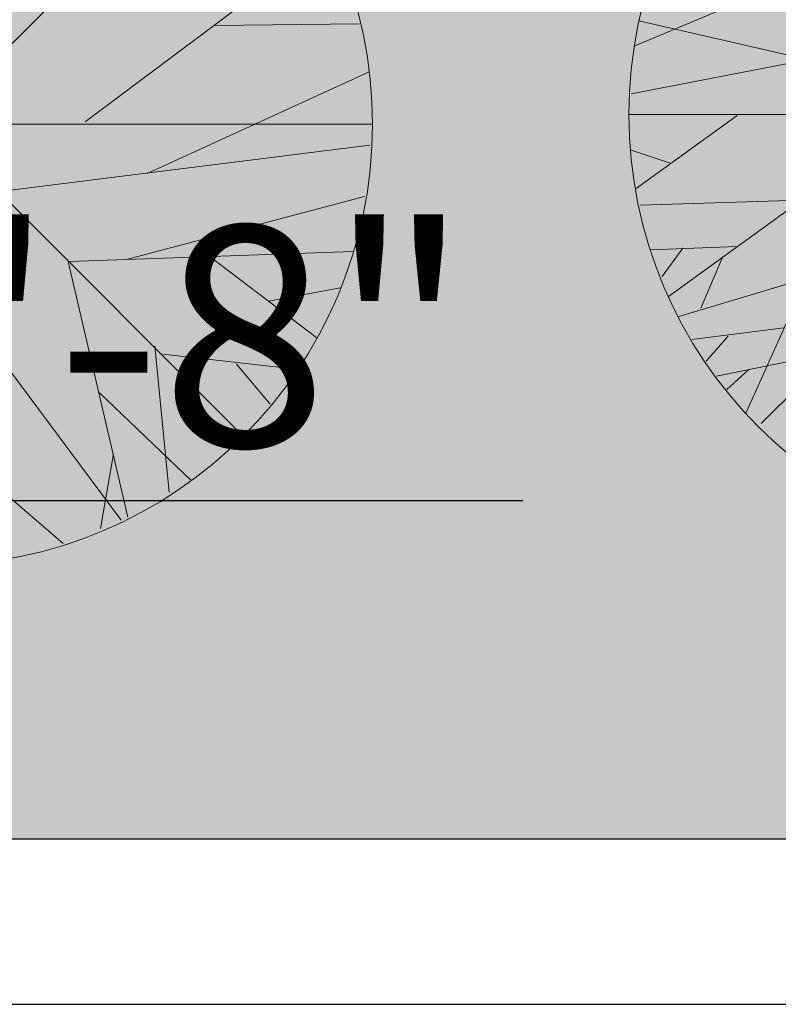
# Model space of a CAD drawing. Units: inches. Extents: x 459864 to 460310, y 324185 to 324787.
# Tile 57 of 112: x 460189 to 460210, y 324195 to 324222. Entities that reach past the tile are written whole.
import ezdxf

# ---------------------------------------------------------------- set-up
doc = ezdxf.new("R2010")
doc.units = ezdxf.units.IN
for name, color, linetype, lineweight in [('A-ANNO-DIMS', 2, 'Continuous', 18), ('C-PROP', 7, 'Continuous', 30), ('L-PLNT', 3, 'Continuous', 13), ('L-SITE-PATT', 252, 'Continuous', 13)]:
    doc.layers.add(name, color=color, linetype=linetype, lineweight=lineweight)
doc.styles.get("Standard").update_dxf_attribs({"font": 'arial.ttf'})
doc.dimstyles.new('ISO-25', dxfattribs={"dimtxt": 6, "dimasz": 2.5, "dimexe": 1.25, "dimexo": 0.625, "dimtad": 1, "dimdec": 1, "dimlunit": 3, "dimtxsty": 'Standard', "dimcen": 2.5, "dimadec": 0, "dimazin": 0, "dimtfac": 1, "dimtdec": 1, "dimtmove": 0, "dimatfit": 3, "dimfxl": 1, "dimarcsym": 0})

# ---------------------------------------------------------------- blocks, each defined once
blk = doc.blocks.new('Tree - deciduous plan')
for p, q in [((42, 42), (-42, -42)), ((42, -42), (-42, 42)), ((54.3626, 25.3731), (20.9119, 0.3198)), ((-32.2571, 20.6333), (-59.1937, 9.348)), ((38.5175, 13.4107), (58.2359, 13.6364)), ((-59.7219, 2.8025), (-12.0106, 12.0565)), ((-58.6656, 12.7336), (-35.9543, 7.5424)), ((29.3626, -6.6771), (59.4682, 7.091)), ((-54.6162, -24.7335), (-20.2853, 0.0941)), ((-60, 0), (60, 0)), ((-45.2853, -0.1316), (-59.0177, -10.0627)), ((9.2922, -9.1598), (59.6443, -2.8401)), ((-59.7219, -4.8714), (-54.2641, -6.6771)), ((26.3697, -18.4138), (58.9401, -9.8369)), ((-58.4895, -12.3197), (-36.4825, -11.6426)), ((-53.2078, -27.442), (-16.7641, -16.6081)), ((18.7992, -18.6394), (57.3556, -17.2853)), ((-57.081, -18.4138), (-45.2853, -17.9624)), ((-52.6797, -18.188), (-55.4966, -22.0251)), ((18.6232, -18.6394), (26.7218, -53.3981)), ((38.1654, -18.188), (52.426, -29.0219)), ((-47.2219, -19.3166), (-50.2148, -26.3135)), ((-0.0388, -19.0909), (25.8415, -53.8495)), ((-35.9543, -22.4765), (-44.0529, -40.5329)), ((45.9119, -24.0564), (55.595, -22.2508)), ((-38.9472, -29.0219), (-51.4472, -30.6018)), ((-46.5177, -30.1504), (-49.5106, -33.536)), ((30.419, -30.1504), (32.3556, -50.0125)), ((31.4753, -31.279), (49.6091, -33.3103)), ((-32.4331, -32.4075), (-48.1021, -35.5674)), ((41.5105, -32.6332), (46.088, -38.0501)), ((-43.7008, -34.6645), (-46.6937, -37.373)), ((-6.2008, -36.2445), (17.919, -57.0094)), ((22.8485, -36.4702), (35.3485, -48.4326)), ((24.7852, -44.8213), (23.0246, -54.978))]:
    blk.add_line(p, q)
blk.add_circle((0, 0), 60)
blk = doc.blocks.new('*D34')
at = {"layer": 'A-ANNO-DIMS', "color": 0, "lineweight": -2, "transparency": 16777216}
for p, q in [((460132.814, 324211.063), (460132.814, 324207.434)), ((460152.838, 324211.063), (460152.838, 324207.434)), ((460135.314, 324208.684), (460150.338, 324208.684)), ((460152.838, 324208.684), (460202.984, 324208.684))]:
    blk.add_line(p, q, dxfattribs=at)
at = {"layer": 'A-ANNO-DIMS', "color": 0, "transparency": 16777216}
for points in [[(460135.314, 324209.101), (460135.314, 324208.268), (460132.814, 324208.684)], [(460150.338, 324209.101), (460150.338, 324208.268), (460152.838, 324208.684)]]:
    blk.add_solid(points, dxfattribs=at)
at = {"layer": 'Defpoints', "color": 0, "transparency": 16777216}
for p in [(460132.814, 324211.688), (460152.838, 324211.688), (460152.838, 324208.684)]:
    blk.add_point(p, dxfattribs=at)
at = {"layer": 'A-ANNO-DIMS', "color": 0, "transparency": 16777216, "insert": (460179.161, 324212.373), "char_height": 6, "attachment_point": 5}
blk.add_mtext('PAVER 1\'-8"', dxfattribs=at)

msp = doc.modelspace()

# ---------------------------------------------------------------- hatches: boundary and pattern name
at = {"layer": 'L-SITE-PATT'}
h = msp.add_hatch(dxfattribs=at)
h.set_pattern_fill('DOTS', color=256)
h.paths.add_polyline_path([(460269.804, 324283.483), (460247.115, 324283.483), (460121.929, 324283.483), (460121.929, 324252.473), (460117.429, 324252.473), (460110.124, 324252.473), (460110.124, 324243.287), (460080.83, 324243.287), (460080.83, 324252.473), (460061.115, 324252.473), (460061.115, 324251.882), (460077.909, 324251.882), (460077.909, 324199.483), (460080.83, 324199.483), (460080.83, 324207.553), (460110.124, 324207.553), (460110.124, 324199.483), (460110.813, 324199.483), (460262.115, 324199.483), (460269.804, 324199.483)], flags=17)
edge = h.paths.add_edge_path(flags=0)
edge.add_ellipse((460222.59, 324263.813), major_axis=(-8.485, 8.485), ratio=1, start_angle=405, end_angle=495, ccw=False)
edge.add_line((460214.821, 324254.66), (460214.832, 324254.666))
edge.add_ellipse((460222.59, 324263.813), major_axis=(-8.485, 8.485), ratio=1, start_angle=405, end_angle=495, ccw=False)
edge.add_line((460210.759, 324261.781), (460210.768, 324261.787))
edge.add_ellipse((460222.59, 324263.813), major_axis=(-8.485, 8.485), ratio=1, start_angle=405, end_angle=495, ccw=False)
edge.add_ellipse((460222.59, 324263.813), major_axis=(-8.485, 8.485), ratio=1, start_angle=392.754, end_angle=405, ccw=False)
edge.add_ellipse((460222.59, 324263.813), major_axis=(-8.485, 8.485), ratio=1, start_angle=380.9347, end_angle=392.754, ccw=False)
edge.add_line((460211.337, 324267.985), (460211.34, 324267.985))
edge.add_ellipse((460222.59, 324263.813), major_axis=(-8.485, 8.485), ratio=1, start_angle=380.9347, end_angle=392.754, ccw=False)
edge.add_ellipse((460222.59, 324263.813), major_axis=(-8.485, 8.485), ratio=1, start_angle=347.9015, end_angle=380.9347, ccw=False)
edge.add_ellipse((460222.59, 324263.813), major_axis=(-8.485, 8.485), ratio=1, start_angle=327.0619, end_angle=347.9015, ccw=False)
edge.add_ellipse((460222.59, 324263.813), major_axis=(-8.485, 8.485), ratio=1, start_angle=278.3246, end_angle=327.0619, ccw=False)
edge.add_line((460225.158, 324275.536), (460225.158, 324275.535))
edge.add_ellipse((460222.59, 324263.813), major_axis=(-8.485, 8.485), ratio=1, start_angle=278.3246, end_angle=327.0619, ccw=False)
edge.add_ellipse((460222.59, 324263.813), major_axis=(-8.485, 8.485), ratio=1, start_angle=260.6436, end_angle=278.3246, ccw=False)
edge.add_ellipse((460222.59, 324263.813), major_axis=(-8.485, 8.485), ratio=1, start_angle=225, end_angle=260.6436, ccw=False)
edge.add_line((460234.509, 324265.243), (460234.501, 324265.239))
edge.add_ellipse((460222.59, 324263.813), major_axis=(-8.485, 8.485), ratio=1, start_angle=225, end_angle=260.6436, ccw=False)
edge.add_ellipse((460222.59, 324263.813), major_axis=(-8.485, 8.485), ratio=1, start_angle=495, end_angle=585, ccw=False)
edge.add_line((460234.437, 324261.861), (460234.424, 324261.858))
edge.add_ellipse((460222.59, 324263.813), major_axis=(-8.485, 8.485), ratio=1, start_angle=495, end_angle=585, ccw=False)
edge.add_line((460227.95, 324253.067), (460227.946, 324253.083))
edge.add_ellipse((460222.59, 324263.813), major_axis=(-8.485, 8.485), ratio=1, start_angle=495, end_angle=585, ccw=False)
edge.add_line((460226.223, 324252.369), (460226.211, 324252.38))
edge.add_ellipse((460222.59, 324263.813), major_axis=(-8.485, 8.485), ratio=1, start_angle=495, end_angle=585, ccw=False)
h.paths.add_polyline_path([(460219.651, 324254.347), (460218.461, 324253.545), (460218.275, 324254.789), (460219.642, 324256.542), (460219.625, 324260.848), (460216.11, 324257.333), (460214.35, 324256.978), (460215.416, 324259.356), (460212.524, 324258.496), (460213.137, 324259.93), (460218.507, 324263.813), (460222.59, 324263.813), (460222.59, 324267.807), (460218.176, 324272.212), (460219.026, 324274.639), (460222.59, 324272.811), (460222.59, 324275.423), (460223.057, 324274.825), (460222.675, 324273.492), (460225.912, 324267.135), (460219.625, 324260.848)], flags=0)
edge = h.paths.add_edge_path(flags=0)
edge.add_ellipse((460194.576, 324264.046), major_axis=(-8.485, 8.485), ratio=1, start_angle=495, end_angle=585, ccw=False)
edge.add_line((460199.936, 324253.3), (460199.932, 324253.316))
edge.add_ellipse((460194.576, 324264.046), major_axis=(-8.485, 8.485), ratio=1, start_angle=495, end_angle=585, ccw=False)
edge.add_line((460198.208, 324252.603), (460198.196, 324252.613))
edge.add_ellipse((460194.576, 324264.046), major_axis=(-8.485, 8.485), ratio=1, start_angle=495, end_angle=585, ccw=False)
edge.add_ellipse((460194.576, 324264.046), major_axis=(-8.485, 8.485), ratio=1, start_angle=405, end_angle=495, ccw=False)
edge.add_line((460186.806, 324254.893), (460186.817, 324254.899))
edge.add_ellipse((460194.576, 324264.046), major_axis=(-8.485, 8.485), ratio=1, start_angle=405, end_angle=495, ccw=False)
edge.add_line((460182.744, 324262.014), (460182.753, 324262.02))
edge.add_ellipse((460194.576, 324264.046), major_axis=(-8.485, 8.485), ratio=1, start_angle=405, end_angle=495, ccw=False)
edge.add_ellipse((460194.576, 324264.046), major_axis=(-8.485, 8.485), ratio=1, start_angle=392.754, end_angle=405, ccw=False)
edge.add_ellipse((460194.576, 324264.046), major_axis=(-8.485, 8.485), ratio=1, start_angle=380.9347, end_angle=392.754, ccw=False)
edge.add_line((460183.323, 324268.218), (460183.326, 324268.218))
edge.add_ellipse((460194.576, 324264.046), major_axis=(-8.485, 8.485), ratio=1, start_angle=380.9347, end_angle=392.754, ccw=False)
edge.add_ellipse((460194.576, 324264.046), major_axis=(-8.485, 8.485), ratio=1, start_angle=347.9015, end_angle=380.9347, ccw=False)
edge.add_ellipse((460194.576, 324264.046), major_axis=(-8.485, 8.485), ratio=1, start_angle=327.0619, end_angle=347.9015, ccw=False)
edge.add_ellipse((460194.576, 324264.046), major_axis=(-8.485, 8.485), ratio=1, start_angle=278.3246, end_angle=327.0619, ccw=False)
edge.add_line((460197.144, 324275.769), (460197.143, 324275.768))
edge.add_ellipse((460194.576, 324264.046), major_axis=(-8.485, 8.485), ratio=1, start_angle=278.3246, end_angle=327.0619, ccw=False)
edge.add_ellipse((460194.576, 324264.046), major_axis=(-8.485, 8.485), ratio=1, start_angle=260.6436, end_angle=278.3246, ccw=False)
edge.add_ellipse((460194.576, 324264.046), major_axis=(-8.485, 8.485), ratio=1, start_angle=225, end_angle=260.6436, ccw=False)
edge.add_line((460206.494, 324265.476), (460206.487, 324265.473))
edge.add_ellipse((460194.576, 324264.046), major_axis=(-8.485, 8.485), ratio=1, start_angle=225, end_angle=260.6436, ccw=False)
edge.add_ellipse((460194.576, 324264.046), major_axis=(-8.485, 8.485), ratio=1, start_angle=495, end_angle=585, ccw=False)
edge.add_line((460206.422, 324262.094), (460206.409, 324262.091))
h.paths.add_polyline_path([(460191.61, 324261.081), (460191.637, 324254.58), (460190.447, 324253.778), (460190.261, 324255.023), (460191.628, 324256.775), (460191.61, 324261.081), (460188.096, 324257.566), (460186.335, 324257.211), (460187.402, 324259.589), (460184.509, 324258.729), (460185.123, 324260.163), (460190.493, 324264.046), (460194.576, 324264.046), (460194.576, 324268.04), (460190.161, 324272.446), (460191.011, 324274.872), (460194.576, 324273.044), (460194.576, 324275.657), (460195.043, 324275.058), (460194.661, 324273.725), (460197.897, 324267.368)], flags=0)
edge = h.paths.add_edge_path(flags=0)
edge.add_ellipse((460252.912, 324263.578), major_axis=(-8.485, 8.485), ratio=1, start_angle=405, end_angle=495, ccw=False)
edge.add_line((460241.081, 324261.545), (460241.089, 324261.551))
edge.add_ellipse((460252.912, 324263.578), major_axis=(-8.485, 8.485), ratio=1, start_angle=405, end_angle=495, ccw=False)
edge.add_ellipse((460252.912, 324263.578), major_axis=(-8.485, 8.485), ratio=1, start_angle=392.754, end_angle=405, ccw=False)
edge.add_ellipse((460252.912, 324263.578), major_axis=(-8.485, 8.485), ratio=1, start_angle=380.9347, end_angle=392.754, ccw=False)
edge.add_line((460241.659, 324267.749), (460241.662, 324267.749))
edge.add_ellipse((460252.912, 324263.578), major_axis=(-8.485, 8.485), ratio=1, start_angle=380.9347, end_angle=392.754, ccw=False)
edge.add_ellipse((460252.912, 324263.578), major_axis=(-8.485, 8.485), ratio=1, start_angle=347.9015, end_angle=380.9347, ccw=False)
edge.add_ellipse((460252.912, 324263.578), major_axis=(-8.485, 8.485), ratio=1, start_angle=327.0619, end_angle=347.9015, ccw=False)
edge.add_ellipse((460252.912, 324263.578), major_axis=(-8.485, 8.485), ratio=1, start_angle=278.3246, end_angle=327.0619, ccw=False)
edge.add_line((460255.48, 324275.3), (460255.479, 324275.299))
edge.add_ellipse((460252.912, 324263.578), major_axis=(-8.485, 8.485), ratio=1, start_angle=278.3246, end_angle=327.0619, ccw=False)
edge.add_ellipse((460252.912, 324263.578), major_axis=(-8.485, 8.485), ratio=1, start_angle=260.6436, end_angle=278.3246, ccw=False)
edge.add_ellipse((460252.912, 324263.578), major_axis=(-8.485, 8.485), ratio=1, start_angle=225, end_angle=260.6436, ccw=False)
edge.add_line((460264.83, 324265.007), (460264.823, 324265.004))
edge.add_ellipse((460252.912, 324263.578), major_axis=(-8.485, 8.485), ratio=1, start_angle=225, end_angle=260.6436, ccw=False)
edge.add_ellipse((460252.912, 324263.578), major_axis=(-8.485, 8.485), ratio=1, start_angle=495, end_angle=585, ccw=False)
edge.add_line((460264.758, 324261.626), (460264.745, 324261.622))
edge.add_ellipse((460252.912, 324263.578), major_axis=(-8.485, 8.485), ratio=1, start_angle=495, end_angle=585, ccw=False)
edge.add_line((460258.272, 324252.832), (460258.268, 324252.848))
edge.add_ellipse((460252.912, 324263.578), major_axis=(-8.485, 8.485), ratio=1, start_angle=495, end_angle=585, ccw=False)
edge.add_line((460256.545, 324252.134), (460256.533, 324252.144))
edge.add_ellipse((460252.912, 324263.578), major_axis=(-8.485, 8.485), ratio=1, start_angle=495, end_angle=585, ccw=False)
edge.add_ellipse((460252.912, 324263.578), major_axis=(-8.485, 8.485), ratio=1, start_angle=405, end_angle=495, ccw=False)
edge.add_line((460245.143, 324254.424), (460245.153, 324254.43))
h.paths.add_polyline_path([(460244.672, 324256.742), (460245.738, 324259.12), (460242.846, 324258.26), (460243.459, 324259.694), (460248.829, 324263.578), (460252.912, 324263.578), (460252.912, 324267.571), (460248.497, 324271.977), (460249.348, 324274.403), (460252.912, 324272.576), (460252.912, 324275.188), (460253.379, 324274.589), (460252.997, 324273.257), (460256.233, 324266.899), (460249.946, 324260.612), (460249.973, 324254.111), (460248.783, 324253.309), (460248.597, 324254.554), (460249.964, 324256.306), (460249.946, 324260.612), (460246.432, 324257.097)], flags=0)
edge = h.paths.add_edge_path(flags=0)
edge.add_ellipse((460167.439, 324262.833), major_axis=(-8.485, 8.485), ratio=1, start_angle=495, end_angle=585, ccw=False)
edge.add_line((460172.799, 324252.087), (460172.795, 324252.103))
edge.add_ellipse((460167.439, 324262.833), major_axis=(-8.485, 8.485), ratio=1, start_angle=495, end_angle=585, ccw=False)
edge.add_line((460171.071, 324251.389), (460171.059, 324251.399))
edge.add_ellipse((460167.439, 324262.833), major_axis=(-8.485, 8.485), ratio=1, start_angle=495, end_angle=585, ccw=False)
edge.add_ellipse((460167.439, 324262.833), major_axis=(-8.485, 8.485), ratio=1, start_angle=405, end_angle=495, ccw=False)
edge.add_line((460159.669, 324253.679), (460159.68, 324253.685))
edge.add_ellipse((460167.439, 324262.833), major_axis=(-8.485, 8.485), ratio=1, start_angle=405, end_angle=495, ccw=False)
edge.add_line((460155.607, 324260.8), (460155.616, 324260.806))
edge.add_ellipse((460167.439, 324262.833), major_axis=(-8.485, 8.485), ratio=1, start_angle=405, end_angle=495, ccw=False)
edge.add_ellipse((460167.439, 324262.833), major_axis=(-8.485, 8.485), ratio=1, start_angle=392.754, end_angle=405, ccw=False)
edge.add_ellipse((460167.439, 324262.833), major_axis=(-8.485, 8.485), ratio=1, start_angle=380.9347, end_angle=392.754, ccw=False)
edge.add_line((460156.185, 324267.005), (460156.189, 324267.005))
edge.add_ellipse((460167.439, 324262.833), major_axis=(-8.485, 8.485), ratio=1, start_angle=380.9347, end_angle=392.754, ccw=False)
edge.add_ellipse((460167.439, 324262.833), major_axis=(-8.485, 8.485), ratio=1, start_angle=347.9015, end_angle=380.9347, ccw=False)
edge.add_ellipse((460167.439, 324262.833), major_axis=(-8.485, 8.485), ratio=1, start_angle=327.0619, end_angle=347.9015, ccw=False)
edge.add_ellipse((460167.439, 324262.833), major_axis=(-8.485, 8.485), ratio=1, start_angle=278.3246, end_angle=327.0619, ccw=False)
edge.add_line((460170.007, 324274.556), (460170.006, 324274.554))
edge.add_ellipse((460167.439, 324262.833), major_axis=(-8.485, 8.485), ratio=1, start_angle=278.3246, end_angle=327.0619, ccw=False)
edge.add_ellipse((460167.439, 324262.833), major_axis=(-8.485, 8.485), ratio=1, start_angle=260.6436, end_angle=278.3246, ccw=False)
edge.add_ellipse((460167.439, 324262.833), major_axis=(-8.485, 8.485), ratio=1, start_angle=225, end_angle=260.6436, ccw=False)
edge.add_line((460179.357, 324264.262), (460179.35, 324264.259))
edge.add_ellipse((460167.439, 324262.833), major_axis=(-8.485, 8.485), ratio=1, start_angle=225, end_angle=260.6436, ccw=False)
edge.add_ellipse((460167.439, 324262.833), major_axis=(-8.485, 8.485), ratio=1, start_angle=495, end_angle=585, ccw=False)
edge.add_line((460179.285, 324260.881), (460179.272, 324260.877))
h.paths.add_polyline_path([(460164.473, 324259.867), (460164.5, 324253.366), (460163.31, 324252.565), (460163.124, 324253.809), (460164.491, 324255.561), (460164.473, 324259.867), (460160.958, 324256.353), (460159.198, 324255.998), (460160.265, 324258.375), (460157.372, 324257.515), (460157.986, 324258.949), (460163.356, 324262.833), (460167.439, 324262.833), (460167.439, 324266.826), (460163.024, 324271.232), (460163.874, 324273.659), (460167.439, 324271.831), (460167.439, 324274.443), (460167.905, 324273.844), (460167.524, 324272.512), (460170.76, 324266.154)], flags=0)
edge = h.paths.add_edge_path(flags=0)
edge.add_ellipse((460140.758, 324262.37), major_axis=(-8.485, 8.485), ratio=1, start_angle=495, end_angle=585, ccw=False)
edge.add_line((460146.118, 324251.624), (460146.114, 324251.639))
edge.add_ellipse((460140.758, 324262.37), major_axis=(-8.485, 8.485), ratio=1, start_angle=495, end_angle=585, ccw=False)
edge.add_line((460144.391, 324250.926), (460144.379, 324250.936))
edge.add_ellipse((460140.758, 324262.37), major_axis=(-8.485, 8.485), ratio=1, start_angle=495, end_angle=585, ccw=False)
edge.add_ellipse((460140.758, 324262.37), major_axis=(-8.485, 8.485), ratio=1, start_angle=405, end_angle=495, ccw=False)
edge.add_line((460132.989, 324253.216), (460132.999, 324253.222))
edge.add_ellipse((460140.758, 324262.37), major_axis=(-8.485, 8.485), ratio=1, start_angle=405, end_angle=495, ccw=False)
edge.add_line((460128.927, 324260.337), (460128.935, 324260.343))
edge.add_ellipse((460140.758, 324262.37), major_axis=(-8.485, 8.485), ratio=1, start_angle=405, end_angle=495, ccw=False)
edge.add_ellipse((460140.758, 324262.37), major_axis=(-8.485, 8.485), ratio=1, start_angle=392.754, end_angle=405, ccw=False)
edge.add_ellipse((460140.758, 324262.37), major_axis=(-8.485, 8.485), ratio=1, start_angle=380.9347, end_angle=392.754, ccw=False)
edge.add_line((460129.505, 324266.541), (460129.508, 324266.541))
edge.add_ellipse((460140.758, 324262.37), major_axis=(-8.485, 8.485), ratio=1, start_angle=380.9347, end_angle=392.754, ccw=False)
edge.add_ellipse((460140.758, 324262.37), major_axis=(-8.485, 8.485), ratio=1, start_angle=347.9015, end_angle=380.9347, ccw=False)
edge.add_ellipse((460140.758, 324262.37), major_axis=(-8.485, 8.485), ratio=1, start_angle=327.0619, end_angle=347.9015, ccw=False)
edge.add_ellipse((460140.758, 324262.37), major_axis=(-8.485, 8.485), ratio=1, start_angle=278.3246, end_angle=327.0619, ccw=False)
edge.add_line((460143.326, 324274.092), (460143.325, 324274.091))
edge.add_ellipse((460140.758, 324262.37), major_axis=(-8.485, 8.485), ratio=1, start_angle=278.3246, end_angle=327.0619, ccw=False)
edge.add_ellipse((460140.758, 324262.37), major_axis=(-8.485, 8.485), ratio=1, start_angle=260.6436, end_angle=278.3246, ccw=False)
edge.add_ellipse((460140.758, 324262.37), major_axis=(-8.485, 8.485), ratio=1, start_angle=225, end_angle=260.6436, ccw=False)
edge.add_line((460152.677, 324263.799), (460152.669, 324263.796))
edge.add_ellipse((460140.758, 324262.37), major_axis=(-8.485, 8.485), ratio=1, start_angle=225, end_angle=260.6436, ccw=False)
edge.add_ellipse((460140.758, 324262.37), major_axis=(-8.485, 8.485), ratio=1, start_angle=495, end_angle=585, ccw=False)
edge.add_line((460152.604, 324260.418), (460152.592, 324260.414))
h.paths.add_polyline_path([(460137.792, 324259.404), (460137.819, 324252.903), (460136.629, 324252.101), (460136.443, 324253.346), (460137.81, 324255.098), (460137.792, 324259.404), (460134.278, 324255.889), (460132.518, 324255.534), (460133.584, 324257.912), (460130.692, 324257.052), (460131.305, 324258.486), (460136.675, 324262.37), (460140.758, 324262.37), (460140.758, 324266.363), (460136.343, 324270.769), (460137.194, 324273.195), (460140.758, 324271.367), (460140.758, 324273.98), (460141.225, 324273.381), (460140.843, 324272.049), (460144.079, 324265.691)], flags=0)
h.paths.add_polyline_path([(460110.124, 324227.414), (460080.83, 324227.414), (460080.83, 324235.484), (460110.124, 324235.484)], flags=16)
h.paths.add_polyline_path([(460110.124, 324220.797), (460110.124, 324212.727), (460080.83, 324212.727), (460080.83, 324220.797)], flags=16)
h.paths.add_polyline_path([(460269.804, 324283.483), (460247.115, 324283.483), (460121.929, 324283.483), (460121.929, 324252.473), (460117.429, 324252.473), (460110.124, 324252.473), (460110.124, 324243.287), (460080.83, 324243.287), (460080.83, 324252.473), (460061.115, 324252.473), (460061.115, 324251.882), (460077.909, 324251.882), (460077.909, 324199.483), (460080.83, 324199.483), (460080.83, 324207.553), (460110.124, 324207.553), (460110.124, 324199.483), (460262.115, 324199.483), (460269.804, 324199.483)], flags=17)
h.paths.add_polyline_path([(460219.651, 324254.347), (460218.461, 324253.545), (460218.275, 324254.789), (460219.642, 324256.542), (460219.625, 324260.848), (460216.11, 324257.333), (460214.35, 324256.978), (460215.416, 324259.356), (460212.524, 324258.496), (460213.137, 324259.93), (460218.507, 324263.813), (460222.59, 324263.813), (460220.18, 324266.223), (460215.461, 324265.308), (460211.835, 324266.137), (460216.247, 324267.985), (460218.418, 324267.985), (460222.59, 324263.813), (460222.59, 324267.807), (460218.176, 324272.212), (460219.026, 324274.639), (460222.59, 324272.811), (460222.59, 324275.423), (460223.057, 324274.825), (460222.675, 324273.492), (460225.912, 324267.135), (460222.59, 324263.813), (460231.383, 324263.813), (460228.485, 324262.488), (460224.425, 324261.978), (460228.68, 324257.724), (460228.966, 324254.791), (460227.142, 324256.537), (460227.542, 324254.819), (460227.333, 324253.614), (460222.59, 324259.985), (460222.59, 324255.497), (460221.377, 324256.541), (460220.576, 324261.799), (460219.625, 324260.848)], flags=0)
h.paths.add_polyline_path([(460199.127, 324256.77), (460199.528, 324255.052), (460199.319, 324253.848), (460194.576, 324260.218), (460194.576, 324255.73), (460193.363, 324256.774), (460192.561, 324262.032), (460191.61, 324261.081), (460191.637, 324254.58), (460190.447, 324253.778), (460190.261, 324255.023), (460191.628, 324256.775), (460191.61, 324261.081), (460188.096, 324257.566), (460186.335, 324257.211), (460187.402, 324259.589), (460184.509, 324258.729), (460185.123, 324260.163), (460190.493, 324264.046), (460194.576, 324264.046), (460192.166, 324266.456), (460187.446, 324265.541), (460183.82, 324266.37), (460188.232, 324268.218), (460190.404, 324268.218), (460194.576, 324264.046), (460194.576, 324268.04), (460190.161, 324272.446), (460191.011, 324274.872), (460194.576, 324273.044), (460194.576, 324275.657), (460195.043, 324275.058), (460194.661, 324273.725), (460197.897, 324267.368), (460194.576, 324264.046), (460203.368, 324264.046), (460200.47, 324262.721), (460196.411, 324262.212), (460200.665, 324257.957), (460200.951, 324255.024)], flags=0)
h.paths.add_polyline_path([(460244.672, 324256.742), (460245.738, 324259.12), (460242.846, 324258.26), (460243.459, 324259.694), (460248.829, 324263.578), (460252.912, 324263.578), (460250.502, 324265.987), (460245.783, 324265.072), (460242.156, 324265.901), (460246.568, 324267.749), (460248.74, 324267.749), (460252.912, 324263.578), (460252.912, 324267.571), (460248.497, 324271.977), (460249.348, 324274.403), (460252.912, 324272.576), (460252.912, 324275.188), (460253.379, 324274.589), (460252.997, 324273.257), (460256.233, 324266.899), (460252.912, 324263.578), (460261.705, 324263.578), (460258.806, 324262.252), (460254.747, 324261.743), (460259.002, 324257.488), (460259.288, 324254.555), (460257.463, 324256.301), (460257.864, 324254.583), (460257.655, 324253.379), (460252.912, 324259.749), (460252.912, 324255.261), (460251.699, 324256.305), (460250.897, 324261.563), (460249.946, 324260.612), (460249.973, 324254.111), (460248.783, 324253.309), (460248.597, 324254.554), (460249.964, 324256.306), (460249.946, 324260.612), (460246.432, 324257.097)], flags=0)
h.paths.add_polyline_path([(460173.528, 324256.743), (460173.814, 324253.811), (460171.99, 324255.556), (460172.39, 324253.838), (460172.182, 324252.634), (460167.439, 324259.004), (460167.439, 324254.516), (460166.226, 324255.56), (460165.424, 324260.818), (460164.473, 324259.867), (460164.5, 324253.366), (460163.31, 324252.565), (460163.124, 324253.809), (460164.491, 324255.561), (460164.473, 324259.867), (460160.958, 324256.353), (460159.198, 324255.998), (460160.265, 324258.375), (460157.372, 324257.515), (460157.986, 324258.949), (460163.356, 324262.833), (460167.439, 324262.833), (460165.029, 324265.243), (460160.309, 324264.327), (460156.683, 324265.156), (460161.095, 324267.005), (460163.267, 324267.005), (460167.439, 324262.833), (460167.439, 324266.826), (460163.024, 324271.232), (460163.874, 324273.659), (460167.439, 324271.831), (460167.439, 324274.443), (460167.905, 324273.844), (460167.524, 324272.512), (460170.76, 324266.154), (460167.439, 324262.833), (460176.231, 324262.833), (460173.333, 324261.507), (460169.274, 324260.998)], flags=0)
h.paths.add_polyline_path([(460146.848, 324256.28), (460147.134, 324253.347), (460145.31, 324255.093), (460145.71, 324253.375), (460145.501, 324252.171), (460140.758, 324258.541), (460140.758, 324254.053), (460139.545, 324255.097), (460138.744, 324260.355), (460137.792, 324259.404), (460137.819, 324252.903), (460136.629, 324252.101), (460136.443, 324253.346), (460137.81, 324255.098), (460137.792, 324259.404), (460134.278, 324255.889), (460132.518, 324255.534), (460133.584, 324257.912), (460130.692, 324257.052), (460131.305, 324258.486), (460136.675, 324262.37), (460140.758, 324262.37), (460138.348, 324264.779), (460133.629, 324263.864), (460130.002, 324264.693), (460134.414, 324266.541), (460136.586, 324266.541), (460140.758, 324262.37), (460140.758, 324266.363), (460136.343, 324270.769), (460137.194, 324273.195), (460140.758, 324271.367), (460140.758, 324273.98), (460141.225, 324273.381), (460140.843, 324272.049), (460144.079, 324265.691), (460140.758, 324262.37), (460149.551, 324262.37), (460146.653, 324261.044), (460142.593, 324260.535)], flags=0)
edge = h.paths.add_edge_path()
edge.add_line((460269.804, 324272.549), (460260.881, 324272.549))
edge.add_ellipse((460252.912, 324263.578), major_axis=(-8.485, 8.485), ratio=1, start_angle=260.6436, end_angle=273.3846, ccw=False)
edge.add_line((460262.283, 324271.092), (460262.261, 324271.091))
edge.add_ellipse((460252.912, 324263.578), major_axis=(-8.485, 8.485), ratio=1, start_angle=260.6436, end_angle=273.3846, ccw=False)
edge.add_ellipse((460252.912, 324263.578), major_axis=(-8.485, 8.485), ratio=1, start_angle=225, end_angle=260.6436, ccw=False)
edge.add_line((460263.609, 324269.063), (460263.572, 324269.058))
edge.add_ellipse((460252.912, 324263.578), major_axis=(-8.485, 8.485), ratio=1, start_angle=225, end_angle=260.6436, ccw=False)
edge.add_line((460264.615, 324266.306), (460264.585, 324266.305))
edge.add_ellipse((460252.912, 324263.578), major_axis=(-8.485, 8.485), ratio=1, start_angle=225, end_angle=260.6436, ccw=False)
edge.add_line((460264.83, 324265.007), (460264.823, 324265.004))
edge.add_ellipse((460252.912, 324263.578), major_axis=(-8.485, 8.485), ratio=1, start_angle=225, end_angle=260.6436, ccw=False)
edge.add_ellipse((460252.912, 324263.578), major_axis=(-8.485, 8.485), ratio=1, start_angle=495, end_angle=585, ccw=False)
edge.add_line((460264.758, 324261.626), (460264.745, 324261.622))
edge.add_ellipse((460252.912, 324263.578), major_axis=(-8.485, 8.485), ratio=1, start_angle=495, end_angle=585, ccw=False)
edge.add_line((460263.442, 324257.739), (460263.389, 324257.779))
edge.add_ellipse((460252.912, 324263.578), major_axis=(-8.485, 8.485), ratio=1, start_angle=495, end_angle=585, ccw=False)
edge.add_line((460258.128, 324252.744), (460258.102, 324252.779))
edge.add_ellipse((460252.912, 324263.578), major_axis=(-8.485, 8.485), ratio=1, start_angle=495, end_angle=585, ccw=False)
edge.add_line((460256.545, 324252.134), (460256.533, 324252.144))
edge.add_ellipse((460252.912, 324263.578), major_axis=(-8.485, 8.485), ratio=1, start_angle=495, end_angle=585, ccw=False)
edge.add_ellipse((460252.912, 324263.578), major_axis=(-8.485, 8.485), ratio=1, start_angle=405, end_angle=495, ccw=False)
edge.add_line((460250.594, 324251.78), (460250.605, 324251.82))
edge.add_ellipse((460252.912, 324263.578), major_axis=(-8.485, 8.485), ratio=1, start_angle=405, end_angle=495, ccw=False)
edge.add_line((460245.143, 324254.424), (460245.153, 324254.43))
edge.add_ellipse((460252.912, 324263.578), major_axis=(-8.485, 8.485), ratio=1, start_angle=405, end_angle=495, ccw=False)
edge.add_line((460243.525, 324256.059), (460243.56, 324256.091))
edge.add_ellipse((460252.912, 324263.578), major_axis=(-8.485, 8.485), ratio=1, start_angle=405, end_angle=495, ccw=False)
edge.add_line((460241.44, 324259.893), (460241.522, 324259.896))
edge.add_ellipse((460252.912, 324263.578), major_axis=(-8.485, 8.485), ratio=1, start_angle=405, end_angle=495, ccw=False)
edge.add_line((460241.081, 324261.545), (460241.089, 324261.551))
edge.add_ellipse((460252.912, 324263.578), major_axis=(-8.485, 8.485), ratio=1, start_angle=405, end_angle=495, ccw=False)
edge.add_ellipse((460252.912, 324263.578), major_axis=(-8.485, 8.485), ratio=1, start_angle=392.754, end_angle=405, ccw=False)
edge.add_line((460241.05, 324265.438), (460241.063, 324265.443))
edge.add_ellipse((460252.912, 324263.578), major_axis=(-8.485, 8.485), ratio=1, start_angle=392.754, end_angle=405, ccw=False)
edge.add_ellipse((460252.912, 324263.578), major_axis=(-8.485, 8.485), ratio=1, start_angle=380.9347, end_angle=392.754, ccw=False)
edge.add_line((460241.452, 324267.176), (460241.469, 324267.171))
edge.add_ellipse((460252.912, 324263.578), major_axis=(-8.485, 8.485), ratio=1, start_angle=380.9347, end_angle=392.754, ccw=False)
edge.add_line((460241.659, 324267.749), (460241.662, 324267.749))
edge.add_ellipse((460252.912, 324263.578), major_axis=(-8.485, 8.485), ratio=1, start_angle=380.9347, end_angle=392.754, ccw=False)
edge.add_ellipse((460252.912, 324263.578), major_axis=(-8.485, 8.485), ratio=1, start_angle=356.6154, end_angle=380.9347, ccw=False)
edge.add_line((460244.88, 324272.488), (460244.713, 324272.549))
edge.add_line((460244.713, 324272.549), (460230.817, 324272.549))
edge.add_ellipse((460222.59, 324263.813), major_axis=(-8.485, 8.485), ratio=1, start_angle=260.6436, end_angle=271.7178, ccw=False)
edge.add_ellipse((460222.59, 324263.813), major_axis=(-8.485, 8.485), ratio=1, start_angle=225, end_angle=260.6436, ccw=False)
edge.add_line((460233.287, 324269.299), (460233.25, 324269.294))
edge.add_ellipse((460222.59, 324263.813), major_axis=(-8.485, 8.485), ratio=1, start_angle=225, end_angle=260.6436, ccw=False)
edge.add_line((460234.294, 324266.541), (460234.264, 324266.541))
edge.add_ellipse((460222.59, 324263.813), major_axis=(-8.485, 8.485), ratio=1, start_angle=225, end_angle=260.6436, ccw=False)
edge.add_line((460234.509, 324265.243), (460234.501, 324265.239))
edge.add_ellipse((460222.59, 324263.813), major_axis=(-8.485, 8.485), ratio=1, start_angle=225, end_angle=260.6436, ccw=False)
edge.add_ellipse((460222.59, 324263.813), major_axis=(-8.485, 8.485), ratio=1, start_angle=495, end_angle=585, ccw=False)
edge.add_line((460234.437, 324261.861), (460234.424, 324261.858))
edge.add_ellipse((460222.59, 324263.813), major_axis=(-8.485, 8.485), ratio=1, start_angle=495, end_angle=585, ccw=False)
edge.add_line((460233.121, 324257.975), (460233.068, 324258.015))
edge.add_ellipse((460222.59, 324263.813), major_axis=(-8.485, 8.485), ratio=1, start_angle=495, end_angle=585, ccw=False)
edge.add_line((460227.806, 324252.979), (460227.78, 324253.014))
edge.add_ellipse((460222.59, 324263.813), major_axis=(-8.485, 8.485), ratio=1, start_angle=495, end_angle=585, ccw=False)
edge.add_line((460226.223, 324252.369), (460226.211, 324252.38))
edge.add_ellipse((460222.59, 324263.813), major_axis=(-8.485, 8.485), ratio=1, start_angle=495, end_angle=585, ccw=False)
edge.add_ellipse((460222.59, 324263.813), major_axis=(-8.485, 8.485), ratio=1, start_angle=405, end_angle=495, ccw=False)
edge.add_line((460220.272, 324252.016), (460220.283, 324252.055))
edge.add_ellipse((460222.59, 324263.813), major_axis=(-8.485, 8.485), ratio=1, start_angle=405, end_angle=495, ccw=False)
edge.add_line((460214.821, 324254.66), (460214.832, 324254.666))
edge.add_ellipse((460222.59, 324263.813), major_axis=(-8.485, 8.485), ratio=1, start_angle=405, end_angle=495, ccw=False)
edge.add_line((460213.203, 324256.295), (460213.239, 324256.327))
edge.add_ellipse((460222.59, 324263.813), major_axis=(-8.485, 8.485), ratio=1, start_angle=405, end_angle=495, ccw=False)
edge.add_line((460211.118, 324260.128), (460211.201, 324260.131))
edge.add_ellipse((460222.59, 324263.813), major_axis=(-8.485, 8.485), ratio=1, start_angle=405, end_angle=495, ccw=False)
edge.add_line((460210.759, 324261.781), (460210.768, 324261.787))
edge.add_ellipse((460222.59, 324263.813), major_axis=(-8.485, 8.485), ratio=1, start_angle=405, end_angle=495, ccw=False)
edge.add_ellipse((460222.59, 324263.813), major_axis=(-8.485, 8.485), ratio=1, start_angle=392.754, end_angle=405, ccw=False)
edge.add_line((460210.729, 324265.673), (460210.741, 324265.678))
edge.add_ellipse((460222.59, 324263.813), major_axis=(-8.485, 8.485), ratio=1, start_angle=392.754, end_angle=405, ccw=False)
edge.add_ellipse((460222.59, 324263.813), major_axis=(-8.485, 8.485), ratio=1, start_angle=380.9347, end_angle=392.754, ccw=False)
edge.add_line((460211.13, 324267.412), (460211.147, 324267.407))
edge.add_ellipse((460222.59, 324263.813), major_axis=(-8.485, 8.485), ratio=1, start_angle=380.9347, end_angle=392.754, ccw=False)
edge.add_line((460211.337, 324267.985), (460211.34, 324267.985))
edge.add_ellipse((460222.59, 324263.813), major_axis=(-8.485, 8.485), ratio=1, start_angle=380.9347, end_angle=392.754, ccw=False)
edge.add_ellipse((460222.59, 324263.813), major_axis=(-8.485, 8.485), ratio=1, start_angle=358.2822, end_angle=380.9347, ccw=False)
edge.add_line((460213.705, 324271.902), (460213.709, 324271.869))
edge.add_ellipse((460222.59, 324263.813), major_axis=(-8.485, 8.485), ratio=1, start_angle=358.2822, end_angle=380.9347, ccw=False)
edge.add_line((460214.363, 324272.549), (460203.078, 324272.549))
edge.add_line((460203.078, 324272.549), (460203.06, 324272.531))
edge.add_ellipse((460194.576, 324264.046), major_axis=(-8.485, 8.485), ratio=1, start_angle=260.6436, end_angle=270.1168, ccw=False)
edge.add_line((460203.957, 324271.561), (460203.921, 324271.56))
edge.add_ellipse((460194.576, 324264.046), major_axis=(-8.485, 8.485), ratio=1, start_angle=260.6436, end_angle=270.1168, ccw=False)
edge.add_ellipse((460194.576, 324264.046), major_axis=(-8.485, 8.485), ratio=1, start_angle=225, end_angle=260.6436, ccw=False)
edge.add_line((460205.272, 324269.532), (460205.235, 324269.527))
edge.add_ellipse((460194.576, 324264.046), major_axis=(-8.485, 8.485), ratio=1, start_angle=225, end_angle=260.6436, ccw=False)
edge.add_line((460206.279, 324266.774), (460206.249, 324266.774))
edge.add_ellipse((460194.576, 324264.046), major_axis=(-8.485, 8.485), ratio=1, start_angle=225, end_angle=260.6436, ccw=False)
edge.add_line((460206.494, 324265.476), (460206.487, 324265.473))
edge.add_ellipse((460194.576, 324264.046), major_axis=(-8.485, 8.485), ratio=1, start_angle=225, end_angle=260.6436, ccw=False)
edge.add_ellipse((460194.576, 324264.046), major_axis=(-8.485, 8.485), ratio=1, start_angle=495, end_angle=585, ccw=False)
edge.add_line((460206.422, 324262.094), (460206.409, 324262.091))
edge.add_ellipse((460194.576, 324264.046), major_axis=(-8.485, 8.485), ratio=1, start_angle=495, end_angle=585, ccw=False)
edge.add_line((460205.106, 324258.208), (460205.053, 324258.248))
edge.add_ellipse((460194.576, 324264.046), major_axis=(-8.485, 8.485), ratio=1, start_angle=495, end_angle=585, ccw=False)
edge.add_line((460199.792, 324253.212), (460199.766, 324253.248))
edge.add_ellipse((460194.576, 324264.046), major_axis=(-8.485, 8.485), ratio=1, start_angle=495, end_angle=585, ccw=False)
edge.add_line((460198.208, 324252.603), (460198.196, 324252.613))
edge.add_ellipse((460194.576, 324264.046), major_axis=(-8.485, 8.485), ratio=1, start_angle=495, end_angle=585, ccw=False)
edge.add_ellipse((460194.576, 324264.046), major_axis=(-8.485, 8.485), ratio=1, start_angle=405, end_angle=495, ccw=False)
edge.add_line((460192.258, 324252.249), (460192.268, 324252.289))
edge.add_ellipse((460194.576, 324264.046), major_axis=(-8.485, 8.485), ratio=1, start_angle=405, end_angle=495, ccw=False)
edge.add_line((460186.806, 324254.893), (460186.817, 324254.899))
edge.add_ellipse((460194.576, 324264.046), major_axis=(-8.485, 8.485), ratio=1, start_angle=405, end_angle=495, ccw=False)
edge.add_line((460185.188, 324256.528), (460185.224, 324256.56))
edge.add_ellipse((460194.576, 324264.046), major_axis=(-8.485, 8.485), ratio=1, start_angle=405, end_angle=495, ccw=False)
edge.add_line((460183.104, 324260.362), (460183.186, 324260.365))
edge.add_ellipse((460194.576, 324264.046), major_axis=(-8.485, 8.485), ratio=1, start_angle=405, end_angle=495, ccw=False)
edge.add_line((460182.744, 324262.014), (460182.753, 324262.02))
edge.add_ellipse((460194.576, 324264.046), major_axis=(-8.485, 8.485), ratio=1, start_angle=405, end_angle=495, ccw=False)
edge.add_ellipse((460194.576, 324264.046), major_axis=(-8.485, 8.485), ratio=1, start_angle=392.754, end_angle=405, ccw=False)
edge.add_line((460182.714, 324265.906), (460182.726, 324265.912))
edge.add_ellipse((460194.576, 324264.046), major_axis=(-8.485, 8.485), ratio=1, start_angle=392.754, end_angle=405, ccw=False)
edge.add_ellipse((460194.576, 324264.046), major_axis=(-8.485, 8.485), ratio=1, start_angle=380.9347, end_angle=392.754, ccw=False)
edge.add_line((460183.116, 324267.645), (460183.133, 324267.64))
edge.add_ellipse((460194.576, 324264.046), major_axis=(-8.485, 8.485), ratio=1, start_angle=380.9347, end_angle=392.754, ccw=False)
edge.add_line((460183.323, 324268.218), (460183.326, 324268.218))
edge.add_ellipse((460194.576, 324264.046), major_axis=(-8.485, 8.485), ratio=1, start_angle=380.9347, end_angle=392.754, ccw=False)
edge.add_ellipse((460194.576, 324264.046), major_axis=(-8.485, 8.485), ratio=1, start_angle=359.8832, end_angle=380.9347, ccw=False)
edge.add_line((460184.491, 324270.611), (460184.553, 324270.611))
edge.add_ellipse((460194.576, 324264.046), major_axis=(-8.485, 8.485), ratio=1, start_angle=359.8832, end_angle=380.9347, ccw=False)
edge.add_line((460185.346, 324271.76), (460185.379, 324271.728))
edge.add_ellipse((460194.576, 324264.046), major_axis=(-8.485, 8.485), ratio=1, start_angle=359.8832, end_angle=380.9347, ccw=False)
edge.add_line((460185.697, 324272.086), (460185.633, 324272.549))
edge.add_line((460185.633, 324272.549), (460174.683, 324272.549))
edge.add_line((460174.683, 324272.549), (460174.606, 324272.457))
edge.add_ellipse((460167.439, 324262.833), major_axis=(-8.485, 8.485), ratio=1, start_angle=260.6436, end_angle=278.3246, ccw=False)
edge.add_ellipse((460167.439, 324262.833), major_axis=(-8.485, 8.485), ratio=1, start_angle=225, end_angle=260.6436, ccw=False)
edge.add_line((460178.135, 324268.318), (460178.098, 324268.313))
edge.add_ellipse((460167.439, 324262.833), major_axis=(-8.485, 8.485), ratio=1, start_angle=225, end_angle=260.6436, ccw=False)
edge.add_line((460179.142, 324265.561), (460179.112, 324265.56))
edge.add_ellipse((460167.439, 324262.833), major_axis=(-8.485, 8.485), ratio=1, start_angle=225, end_angle=260.6436, ccw=False)
edge.add_line((460179.357, 324264.262), (460179.35, 324264.259))
edge.add_ellipse((460167.439, 324262.833), major_axis=(-8.485, 8.485), ratio=1, start_angle=225, end_angle=260.6436, ccw=False)
edge.add_ellipse((460167.439, 324262.833), major_axis=(-8.485, 8.485), ratio=1, start_angle=495, end_angle=585, ccw=False)
edge.add_line((460179.285, 324260.881), (460179.272, 324260.877))
edge.add_ellipse((460167.439, 324262.833), major_axis=(-8.485, 8.485), ratio=1, start_angle=495, end_angle=585, ccw=False)
edge.add_line((460177.969, 324256.994), (460177.916, 324257.034))
edge.add_ellipse((460167.439, 324262.833), major_axis=(-8.485, 8.485), ratio=1, start_angle=495, end_angle=585, ccw=False)
edge.add_line((460172.655, 324251.999), (460172.629, 324252.034))
edge.add_ellipse((460167.439, 324262.833), major_axis=(-8.485, 8.485), ratio=1, start_angle=495, end_angle=585, ccw=False)
edge.add_line((460171.071, 324251.389), (460171.059, 324251.399))
edge.add_ellipse((460167.439, 324262.833), major_axis=(-8.485, 8.485), ratio=1, start_angle=495, end_angle=585, ccw=False)
edge.add_ellipse((460167.439, 324262.833), major_axis=(-8.485, 8.485), ratio=1, start_angle=405, end_angle=495, ccw=False)
edge.add_line((460165.121, 324251.036), (460165.131, 324251.075))
edge.add_ellipse((460167.439, 324262.833), major_axis=(-8.485, 8.485), ratio=1, start_angle=405, end_angle=495, ccw=False)
edge.add_line((460159.669, 324253.679), (460159.68, 324253.685))
edge.add_ellipse((460167.439, 324262.833), major_axis=(-8.485, 8.485), ratio=1, start_angle=405, end_angle=495, ccw=False)
edge.add_line((460158.051, 324255.314), (460158.087, 324255.347))
edge.add_ellipse((460167.439, 324262.833), major_axis=(-8.485, 8.485), ratio=1, start_angle=405, end_angle=495, ccw=False)
edge.add_line((460155.967, 324259.148), (460156.049, 324259.151))
edge.add_ellipse((460167.439, 324262.833), major_axis=(-8.485, 8.485), ratio=1, start_angle=405, end_angle=495, ccw=False)
edge.add_line((460155.607, 324260.8), (460155.616, 324260.806))
edge.add_ellipse((460167.439, 324262.833), major_axis=(-8.485, 8.485), ratio=1, start_angle=405, end_angle=495, ccw=False)
edge.add_ellipse((460167.439, 324262.833), major_axis=(-8.485, 8.485), ratio=1, start_angle=392.754, end_angle=405, ccw=False)
edge.add_line((460155.577, 324264.693), (460155.589, 324264.698))
edge.add_ellipse((460167.439, 324262.833), major_axis=(-8.485, 8.485), ratio=1, start_angle=392.754, end_angle=405, ccw=False)
edge.add_ellipse((460167.439, 324262.833), major_axis=(-8.485, 8.485), ratio=1, start_angle=380.9347, end_angle=392.754, ccw=False)
edge.add_line((460155.979, 324266.432), (460155.996, 324266.426))
edge.add_ellipse((460167.439, 324262.833), major_axis=(-8.485, 8.485), ratio=1, start_angle=380.9347, end_angle=392.754, ccw=False)
edge.add_line((460156.185, 324267.005), (460156.189, 324267.005))
edge.add_ellipse((460167.439, 324262.833), major_axis=(-8.485, 8.485), ratio=1, start_angle=380.9347, end_angle=392.754, ccw=False)
edge.add_ellipse((460167.439, 324262.833), major_axis=(-8.485, 8.485), ratio=1, start_angle=350.9345, end_angle=380.9347, ccw=False)
edge.add_line((460157.363, 324269.397), (460157.414, 324269.397))
edge.add_ellipse((460167.439, 324262.833), major_axis=(-8.485, 8.485), ratio=1, start_angle=350.9345, end_angle=380.9347, ccw=False)
edge.add_line((460158.221, 324270.535), (460158.236, 324270.519))
edge.add_ellipse((460167.439, 324262.833), major_axis=(-8.485, 8.485), ratio=1, start_angle=350.9345, end_angle=380.9347, ccw=False)
edge.add_line((460159.379, 324271.753), (460159.419, 324271.738))
edge.add_ellipse((460167.439, 324262.833), major_axis=(-8.485, 8.485), ratio=1, start_angle=350.9345, end_angle=380.9347, ccw=False)
edge.add_line((460160.396, 324272.549), (460147.112, 324272.549))
edge.add_ellipse((460140.758, 324262.37), major_axis=(-8.485, 8.485), ratio=1, start_angle=278.3246, end_angle=283.0261, ccw=False)
edge.add_ellipse((460140.758, 324262.37), major_axis=(-8.485, 8.485), ratio=1, start_angle=260.6436, end_angle=278.3246, ccw=False)
edge.add_ellipse((460140.758, 324262.37), major_axis=(-8.485, 8.485), ratio=1, start_angle=225, end_angle=260.6436, ccw=False)
edge.add_line((460151.455, 324267.855), (460151.418, 324267.85))
edge.add_ellipse((460140.758, 324262.37), major_axis=(-8.485, 8.485), ratio=1, start_angle=225, end_angle=260.6436, ccw=False)
edge.add_line((460152.462, 324265.098), (460152.431, 324265.097))
edge.add_ellipse((460140.758, 324262.37), major_axis=(-8.485, 8.485), ratio=1, start_angle=225, end_angle=260.6436, ccw=False)
edge.add_line((460152.677, 324263.799), (460152.669, 324263.796))
edge.add_ellipse((460140.758, 324262.37), major_axis=(-8.485, 8.485), ratio=1, start_angle=225, end_angle=260.6436, ccw=False)
edge.add_ellipse((460140.758, 324262.37), major_axis=(-8.485, 8.485), ratio=1, start_angle=495, end_angle=585, ccw=False)
edge.add_line((460152.604, 324260.418), (460152.592, 324260.414))
edge.add_ellipse((460140.758, 324262.37), major_axis=(-8.485, 8.485), ratio=1, start_angle=495, end_angle=585, ccw=False)
edge.add_line((460151.288, 324256.531), (460151.235, 324256.571))
edge.add_ellipse((460140.758, 324262.37), major_axis=(-8.485, 8.485), ratio=1, start_angle=495, end_angle=585, ccw=False)
edge.add_line((460145.974, 324251.535), (460145.948, 324251.571))
edge.add_ellipse((460140.758, 324262.37), major_axis=(-8.485, 8.485), ratio=1, start_angle=495, end_angle=585, ccw=False)
edge.add_line((460144.391, 324250.926), (460144.379, 324250.936))
edge.add_ellipse((460140.758, 324262.37), major_axis=(-8.485, 8.485), ratio=1, start_angle=495, end_angle=585, ccw=False)
edge.add_ellipse((460140.758, 324262.37), major_axis=(-8.485, 8.485), ratio=1, start_angle=405, end_angle=495, ccw=False)
edge.add_line((460138.44, 324250.572), (460138.451, 324250.612))
edge.add_ellipse((460140.758, 324262.37), major_axis=(-8.485, 8.485), ratio=1, start_angle=405, end_angle=495, ccw=False)
edge.add_line((460132.989, 324253.216), (460132.999, 324253.222))
edge.add_ellipse((460140.758, 324262.37), major_axis=(-8.485, 8.485), ratio=1, start_angle=405, end_angle=495, ccw=False)
edge.add_line((460131.371, 324254.851), (460131.406, 324254.883))
edge.add_ellipse((460140.758, 324262.37), major_axis=(-8.485, 8.485), ratio=1, start_angle=405, end_angle=495, ccw=False)
edge.add_line((460129.286, 324258.685), (460129.369, 324258.688))
edge.add_ellipse((460140.758, 324262.37), major_axis=(-8.485, 8.485), ratio=1, start_angle=405, end_angle=495, ccw=False)
edge.add_line((460128.927, 324260.337), (460128.935, 324260.343))
edge.add_ellipse((460140.758, 324262.37), major_axis=(-8.485, 8.485), ratio=1, start_angle=405, end_angle=495, ccw=False)
edge.add_ellipse((460140.758, 324262.37), major_axis=(-8.485, 8.485), ratio=1, start_angle=392.754, end_angle=405, ccw=False)
edge.add_line((460128.896, 324264.23), (460128.909, 324264.235))
edge.add_ellipse((460140.758, 324262.37), major_axis=(-8.485, 8.485), ratio=1, start_angle=392.754, end_angle=405, ccw=False)
edge.add_ellipse((460140.758, 324262.37), major_axis=(-8.485, 8.485), ratio=1, start_angle=380.9347, end_angle=392.754, ccw=False)
edge.add_line((460129.298, 324265.968), (460129.315, 324265.963))
edge.add_ellipse((460140.758, 324262.37), major_axis=(-8.485, 8.485), ratio=1, start_angle=380.9347, end_angle=392.754, ccw=False)
edge.add_line((460129.505, 324266.541), (460129.508, 324266.541))
edge.add_ellipse((460140.758, 324262.37), major_axis=(-8.485, 8.485), ratio=1, start_angle=380.9347, end_angle=392.754, ccw=False)
edge.add_ellipse((460140.758, 324262.37), major_axis=(-8.485, 8.485), ratio=1, start_angle=347.9015, end_angle=380.9347, ccw=False)
edge.add_line((460130.697, 324268.934), (460130.727, 324268.934))
edge.add_ellipse((460140.758, 324262.37), major_axis=(-8.485, 8.485), ratio=1, start_angle=347.9015, end_angle=380.9347, ccw=False)
edge.add_line((460131.869, 324270.48), (460131.879, 324270.413))
edge.add_ellipse((460140.758, 324262.37), major_axis=(-8.485, 8.485), ratio=1, start_angle=347.9015, end_angle=380.9347, ccw=False)
edge.add_line((460132.734, 324271.277), (460132.705, 324271.287))
edge.add_ellipse((460140.758, 324262.37), major_axis=(-8.485, 8.485), ratio=1, start_angle=347.9015, end_angle=380.9347, ccw=False)
edge.add_line((460134.24, 324272.445), (460134.204, 324272.549))
edge.add_line((460134.204, 324272.549), (460121.929, 324272.549))
edge.add_line((460121.929, 324272.549), (460121.929, 324252.473))
edge.add_line((460121.929, 324252.473), (460117.429, 324252.473))
edge.add_line((460117.429, 324252.473), (460110.124, 324252.473))
edge.add_line((460110.124, 324252.473), (460110.124, 324243.287))
edge.add_line((460110.124, 324243.287), (460080.83, 324243.287))
edge.add_line((460080.83, 324243.287), (460080.83, 324252.473))
edge.add_line((460080.83, 324252.473), (460061.115, 324252.473))
edge.add_line((460061.115, 324252.473), (460061.115, 324251.882))
edge.add_line((460061.115, 324251.882), (460077.909, 324251.882))
edge.add_line((460077.909, 324251.882), (460077.909, 324199.483))
edge.add_line((460077.909, 324199.483), (460080.83, 324199.483))
edge.add_line((460080.83, 324199.483), (460080.83, 324207.553))
edge.add_line((460080.83, 324207.553), (460110.124, 324207.553))
edge.add_line((460110.124, 324207.553), (460110.124, 324199.483))
edge.add_line((460110.124, 324199.483), (460110.813, 324199.483))
edge.add_line((460110.813, 324199.483), (460262.115, 324199.483))
edge.add_line((460262.115, 324199.483), (460269.804, 324199.483))
edge.add_line((460269.804, 324199.483), (460269.804, 324272.549))

# ---------------------------------------------------------------- linework, layer by layer
at = {"layer": 'C-PROP'}
for p, q in [((460061.115, 324199.483), (460262.115, 324199.483)), ((460061.115, 324194.983), (460271.115, 324194.983))]:
    msp.add_line(p, q, dxfattribs=at)

# ---------------------------------------------------------------- block references
at = {"layer": 'L-PLNT', "xscale": 0.2, "yscale": 0.2}
for p in [(460217.87, 324219.178), (460186.892, 324218.913)]:
    msp.add_blockref('Tree - deciduous plan', p, dxfattribs=at)

# ---------------------------------------------------------------- dimensions: what is measured, and where the dimension line sits
at = {"layer": 'A-ANNO-DIMS'}
dim = msp.add_linear_dim(base=(460152.838, 324208.684), p1=(460132.814, 324211.688), p2=(460152.838, 324211.688), text='PAVER <>', dimstyle='ISO-25', override={"dimdec": 1, "dimlfac": 1, "dimrnd": 0, "dimzin": 1, "dimdsep": 46, "dimlunit": 4, "dimfrac": 2}, dxfattribs=at)
dim.commit()
dim.dimension.update_dxf_attribs({"geometry": '*D34', "text_midpoint": (460179.161, 324212.373)})

doc.saveas('drawing.dxf')
